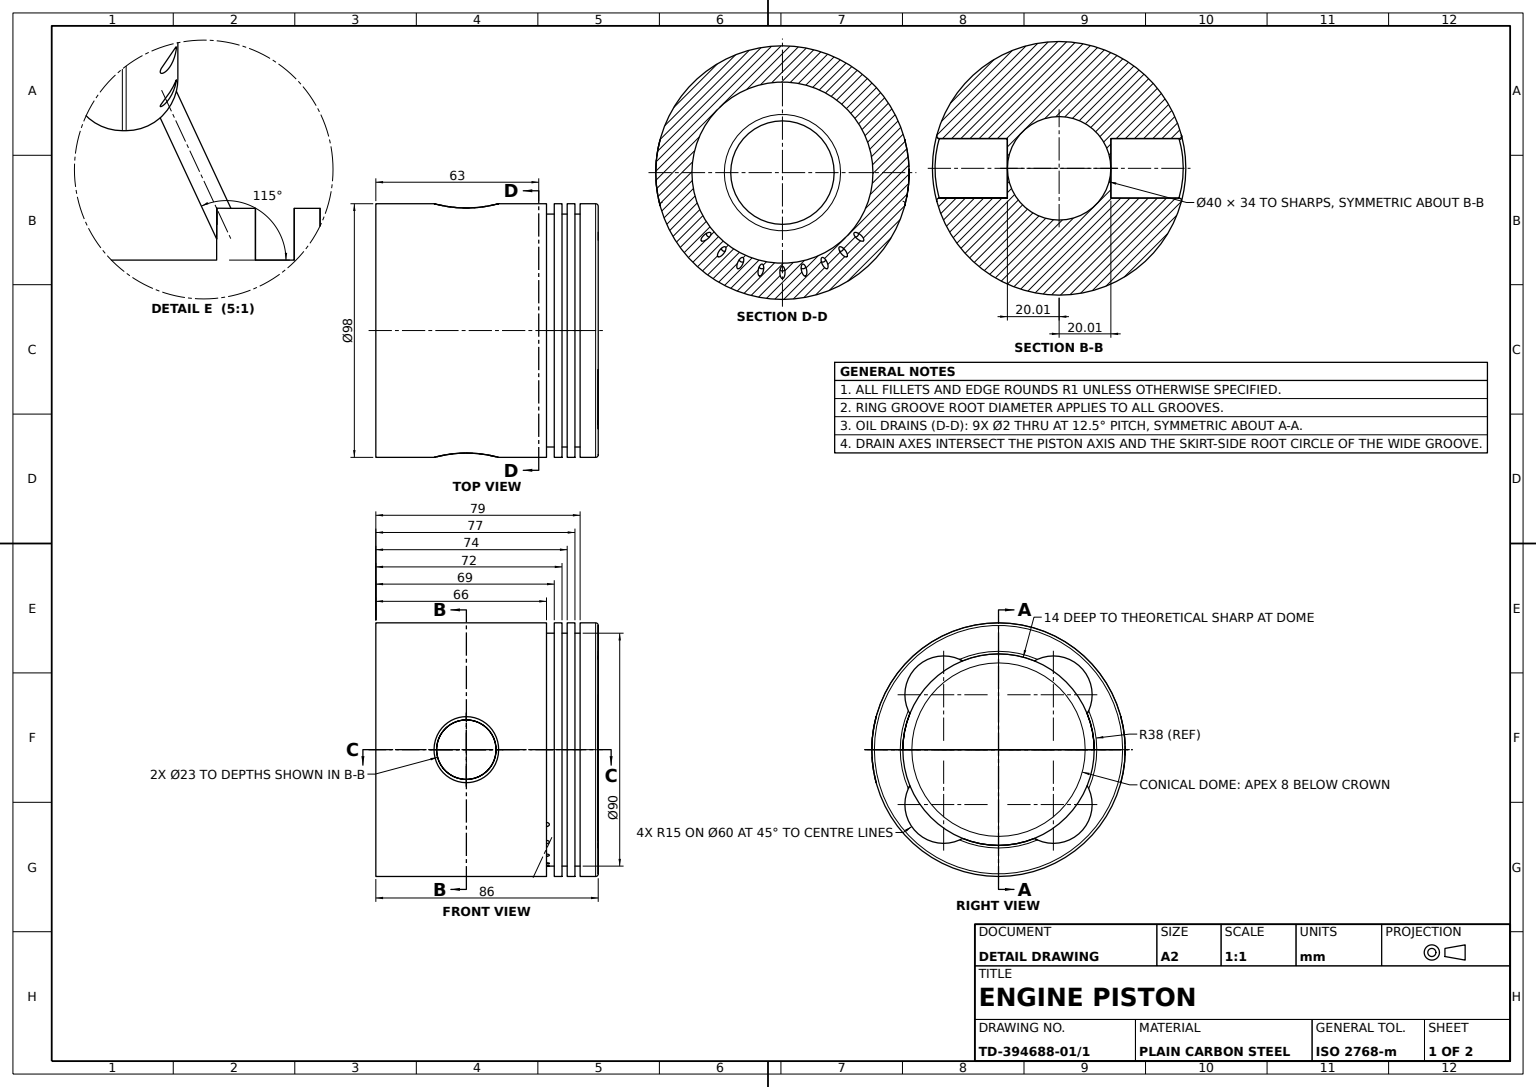
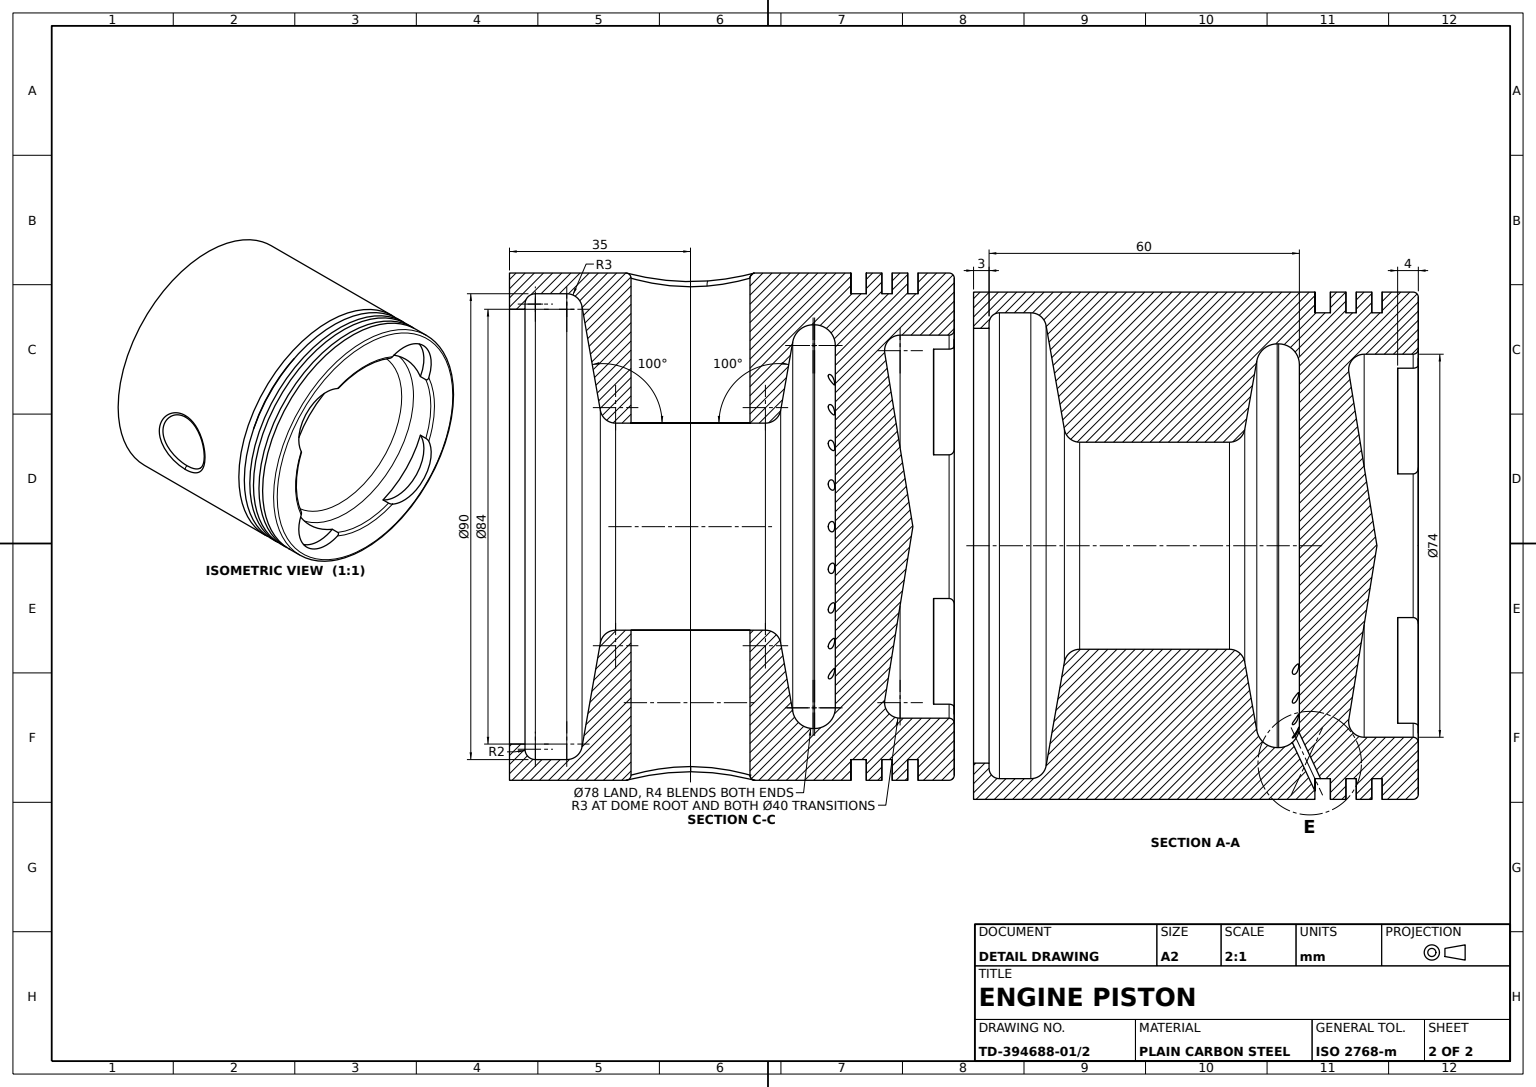
from build123d import *
from OCP.BRepFilletAPI import BRepFilletAPI_MakeFillet

# Parameters (mm, degrees)
INTERNAL_CAVITY_FILLET_R4_R             = 4
PIN_BORE_CUT_REACH                      = 132.455
PIN_BORE_CUT_END_RADIUS                 = 49
PIN_START                               = 20.01
PIN_BORE_SKETCH_R                       = 11.5
CROWN_RECESS_SKETCH_R                   = 37
CROWN_RECESS_CUT_DEPTH                  = 14
CROWN_RECESS_FILLETS_R1                 = 1
CROWN_RECESS_FILLETS_R2                 = 3
PIN_BORE_EDGE_FILLET_R1_R               = 1
VALVE_RELIEFS_CUT_DEPTH                 = 4
OIL_HOLE_PATTERN_5X_COUNT               = 5
OIL_HOLE_PATTERN_5X_ANGLE               = 50
OIL_HOLE_PATTERN_5X_THE_OTHER_WAY_COUNT = 5
OIL_HOLE_PATTERN_5X_THE_OTHER_WAY_ANGLE = 50


with BuildPart() as part:
    # Piston Body Profile → Piston Body (revolve)
    with BuildSketch(Plane(origin=(0, 0, 0), x_dir=(0, 0, -1), z_dir=(1, 0, 0)), mode=Mode.PRIVATE) as piston_body_sk:
        Polygon((0, 0), (-49, 0), (-49, 66), (-45, 66), (-45, 69), (-49, 69), (-49, 72), (-45, 72), (-45, 74), (-49, 74), (-49, 77), (-45, 77), (-45, 79), (-49, 79), (-49, 86), (0, 86), align=None)
    revolve(piston_body_sk.sketch.rotate(Axis((0, 0, 0), (0, 1, 0)), 180), axis=Axis((0, 0, 0), (0, 1, 0)))

    # Internal Cavity Profile → Internal Cooling Cavity Cut (revolve, cut)
    with BuildSketch(Plane(origin=(0, 0, 0), x_dir=(0, 0, -1), z_dir=(1, 0, 0)), mode=Mode.PRIVATE) as internal_cooling_cavity_cut_sk:
        with BuildLine():
            Line((-42, 0), (-42, 3))
            Line((-42, 3), (-43, 3))
            ThreePointArc((-43, 3), (-44.414213562, 3.585786438), (-45, 5))
            Line((-45, 5), (-45, 11.074526589))
            ThreePointArc((-45, 11.074526589), (-44.298133329, 13.002889418), (-42.520944533, 14.028949848))
            Line((-42.520944533, 14.028949848), (-22.479055467, 17.562875634))
            ThreePointArc((-22.479055467, 17.562875634), (-20.701866671, 18.588936064), (-20, 20.517298894))
            Line((-20, 20.517298894), (-20, 49.482701106))
            ThreePointArc((-20, 49.482701106), (-20.701866671, 51.411063936), (-22.479055467, 52.437124366))
            Line((-22.479055467, 52.437124366), (-39, 55.350212633))
            Line((-39, 55.350212633), (-39, 63))
            Line((-39, 63), (0, 63))
            Line((0, 63), (0, 0))
            Line((0, 0), (-42, 0))
        make_face()
    revolve(internal_cooling_cavity_cut_sk.sketch.rotate(Axis((0, 0, 0), (0, 1, 0)), 180), axis=Axis((0, 0, 0), (0, 1, 0)), mode=Mode.SUBTRACT)

    # Internal Cavity Fillet R4
    internal_cavity_fillet_r4_edges = [part.edges().sort_by_distance(p)[0] for p in [
        (0, 63, 39),
        (0, 55.350212633, 39),
    ]]
    fillet(internal_cavity_fillet_r4_edges, radius=INTERNAL_CAVITY_FILLET_R4_R)

    # Pin Bore Cut: up to this cylinder (the profile starts inside it)
    pin_bore_cut_end = Plane(origin=(0, 35, 0), z_dir=(0, -1, 0)) * Cylinder(PIN_BORE_CUT_END_RADIUS, 363.91, mode=Mode.PRIVATE)
    # Pin Bore Sketch → Pin Bore Cut (cut, up to the surface)
    with BuildSketch(Plane.XY.offset(PIN_START), mode=Mode.PRIVATE) as pin_bore_cut_sk1:
        with Locations(Location((0, 35, 0), (0, 0, 180))):
            Circle(PIN_BORE_SKETCH_R)
    pin_bore_cut_tool1 = extrude(pin_bore_cut_sk1.sketch, amount=PIN_BORE_CUT_REACH, mode=Mode.PRIVATE) & pin_bore_cut_end
    pin_bore_cut = pin_bore_cut_tool1.solids().sort_by_distance((0, 35, 20.01))[0]
    add(pin_bore_cut, mode=Mode.SUBTRACT)

    # Pin Bore Mirror: Pin Bore Cut across plane
    add(pin_bore_cut.mirror(Plane.XY), mode=Mode.SUBTRACT)

    # Crown Recess Sketch → Crown Recess Cut (cut)
    with BuildSketch(Plane(origin=(0, 86, 0), x_dir=(1, 0, 0), z_dir=(0, 1, 0))):
        with Locations(Location((0, 0, 0), (0, 0, 270))):
            Circle(CROWN_RECESS_SKETCH_R)
    extrude(amount=-CROWN_RECESS_CUT_DEPTH, mode=Mode.SUBTRACT)

    # Crown Dome Profile → Crown Dome (revolve)
    with BuildSketch(Plane(origin=(0, 0, 0), x_dir=(0, 0, -1), z_dir=(1, 0, 0)), mode=Mode.PRIVATE) as crown_dome_sk:
        Polygon((0, 78), (-37, 72), (0, 72), align=None)
    revolve(crown_dome_sk.sketch.rotate(Axis((0, 86, 0), (0, -1, 0)), 180), axis=Axis((0, 86, 0), (0, -1, 0)))

    # Crown Recess Fillets: one fillet with a radius per group of edges: ONE call of the kernel's fillet builder (fillet() takes one radius for all edges)
    crown_recess_fillets_edges_1 = [part.edges().sort_by_distance(p)[0] for p in [
        (0, 86, -37),
        (0, 86, 49),
    ]]
    crown_recess_fillets_edges_2 = [part.edges().sort_by_distance(p)[0] for p in [
        (-37, 72, 0),
    ]]
    crown_recess_fillets = BRepFilletAPI_MakeFillet(part.part.solid().wrapped)
    for e in crown_recess_fillets_edges_1:
        crown_recess_fillets.Add(CROWN_RECESS_FILLETS_R1, e.wrapped)
    for e in crown_recess_fillets_edges_2:
        crown_recess_fillets.Add(CROWN_RECESS_FILLETS_R2, e.wrapped)
    add(Compound.cast(crown_recess_fillets.Shape()), mode=Mode.REPLACE)

    # Pin Bore Edge Fillet R1
    pin_bore_edge_fillet_r1_edges = [part.edges().sort_by_distance(p)[0] for p in [
        (11.5, 35, 47.631397208),
        (-8.131996782, 43.131459181, -48.320499049),
    ]]
    fillet(pin_bore_edge_fillet_r1_edges, radius=PIN_BORE_EDGE_FILLET_R1_R)

    # Sketch5_3 → Valve Reliefs Cut (cut)
    with BuildSketch(Plane(origin=(0, 86, 0), x_dir=(1, 0, 0), z_dir=(0, 1, 0))):
        with BuildLine():
            ThreePointArc((-34.298134906, -13.879407119), (-31.819805153, -31.819805153), (-13.879407119, -34.298134906))
            ThreePointArc((-13.879407119, -34.298134906), (-26.162950904, -26.162950904), (-34.298134906, -13.879407119))
        make_face()
        with BuildLine():
            ThreePointArc((-34.298134906, 13.879407119), (-26.162950904, 26.162950904), (-13.879407119, 34.298134906))
            ThreePointArc((-13.879407119, 34.298134906), (-31.819805153, 31.819805153), (-34.298134906, 13.879407119))
        make_face()
        with BuildLine():
            ThreePointArc((13.879407119, 34.298134906), (26.162950904, 26.162950904), (34.298134906, 13.879407119))
            ThreePointArc((34.298134906, 13.879407119), (31.819805153, 31.819805153), (13.879407119, 34.298134906))
        make_face()
        with BuildLine():
            ThreePointArc((13.879407119, -34.298134906), (31.819805153, -31.819805153), (34.298134906, -13.879407119))
            ThreePointArc((34.298134906, -13.879407119), (26.162950904, -26.162950904), (13.879407119, -34.298134906))
        make_face()
    extrude(amount=-VALVE_RELIEFS_CUT_DEPTH, mode=Mode.SUBTRACT)

    # Oil Hole Profile → Oil Hole Cut (revolve, cut)
    with BuildSketch(Plane.XY, mode=Mode.PRIVATE) as oil_hole_cut_sk:
        Polygon((36.020386059, 60.709359333), (48.708193481, 66.625781099), (48.285575219, 67.532088886), (35.597767797, 61.61566712), align=None)
    oil_hole_cut = revolve(oil_hole_cut_sk.sketch.rotate(Axis((48.285575219, 67.532088886, 0), (-0.9063077870366514, -0.4226182617406964, 0)), 192.922852053), axis=Axis((48.285575219, 67.532088886, 0), (-0.9063077870366514, -0.4226182617406964, 0)), mode=Mode.SUBTRACT)

    # Oil Hole Pattern 5x: Oil Hole Cut ×5 about axis
    oil_hole_pattern_5x_axis = Axis((0, 78, 0), (0, -1, 0))
    for i in range(1, OIL_HOLE_PATTERN_5X_COUNT):
        add(oil_hole_cut.rotate(oil_hole_pattern_5x_axis, i * OIL_HOLE_PATTERN_5X_ANGLE / (OIL_HOLE_PATTERN_5X_COUNT - 1)), mode=Mode.SUBTRACT)

    # Oil Hole Pattern 5x the other way: Oil Hole Cut ×5 about axis
    oil_hole_pattern_5x_the_other_way_axis = Axis((0, 78, 0), (0, 1, 0))
    for i in range(1, OIL_HOLE_PATTERN_5X_THE_OTHER_WAY_COUNT):
        add(oil_hole_cut.rotate(oil_hole_pattern_5x_the_other_way_axis, i * OIL_HOLE_PATTERN_5X_THE_OTHER_WAY_ANGLE / (OIL_HOLE_PATTERN_5X_THE_OTHER_WAY_COUNT - 1)), mode=Mode.SUBTRACT)


solid = part.part
